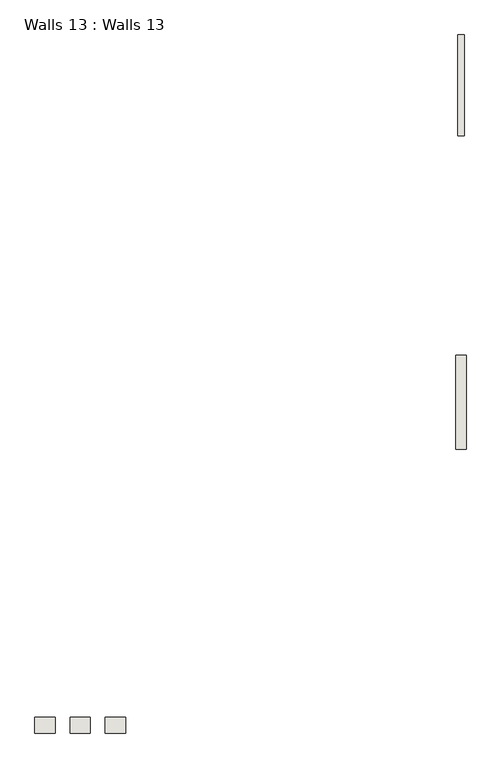
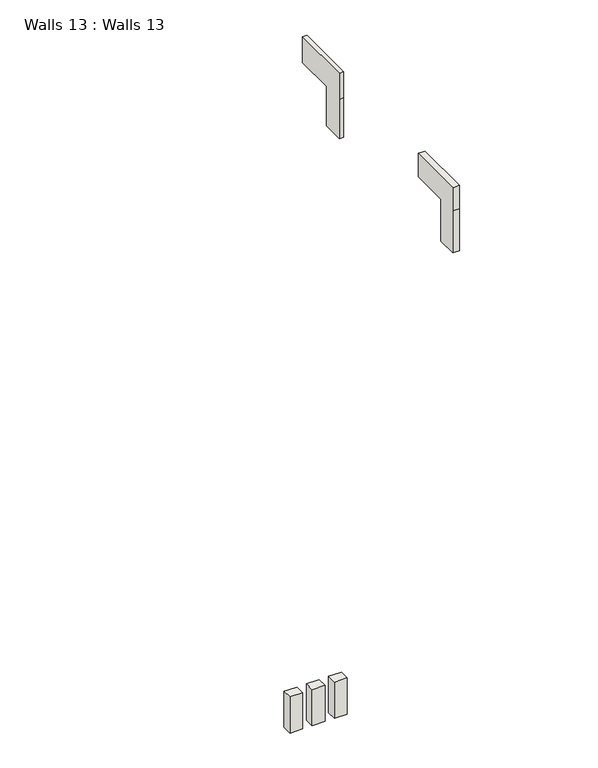
"""IFC4 building model written with IfcOpenShell, lengths in millimetres: wall geometry, Walls 13 : Walls 13."""

from ifc_helpers import new_model, si_unit, frame, origin, place, context, project, spatial, polyline, outline, extrude, source, transform, mapped, element, save


def walls_13_walls_13_75e322be(model_context):
    return source(origin(), model_context, "Body", "SweptSolid", [
        extrude(outline(polyline([(5900.1740351, 9474.2), (5900.1740351, 8820.1275419), (4918.9383511, 8820.1275419), (4918.9383511, 7820.7521516), (4376.1740351, 7820.7521516), (4376.1740351, 8820.1275419), (4376.1740351, 9474.2), (5900.1740351, 9474.2)])), frame((2302.6685091, 0.0, 0.0), z_axis=(1.0, 0.0, 0.0), x_axis=(0.0, 1.0, 0.0)), (0.0, 0.0, 1.0), 101.8221291),
        extrude(outline(polyline([(1048.7740351, 9474.2), (1048.7740351, 8885.7171315), (120.9450154, 8885.7171315), (120.9450154, 7820.7521516), (-373.6259649, 7820.7521516), (-373.6259649, 8885.7171315), (-373.6259649, 9474.2), (1048.7740351, 9474.2)])), frame((2272.4271302, 0.0, 0.0), z_axis=(1.0, 0.0, 0.0), x_axis=(0.0, 1.0, 0.0)), (0.0, 0.0, 1.0), 157.4776868),
        extrude(outline(polyline([(-3798.4727244, -4666.7213241), (-4103.2727244, -4666.7213241), (-4103.2727244, -4430.287454), (-3798.4727244, -4430.287454), (-3798.4727244, -4666.7213241)])), frame((0.0, 0.0, 519.7613395), z_axis=(0.0, 0.0, 1.0), x_axis=(1.0, 0.0, 0.0)), (0.0, 0.0, 1.0), 914.4),
        extrude(outline(polyline([(-3265.0727244, -4666.7213241), (-3569.8727244, -4666.7213241), (-3569.8727244, -4430.287454), (-3265.0727244, -4430.287454), (-3265.0727244, -4666.7213241)])), frame((0.0, 0.0, 519.7613395), z_axis=(0.0, 0.0, 1.0), x_axis=(1.0, 0.0, 0.0)), (0.0, 0.0, 1.0), 914.4),
        extrude(outline(polyline([(-2731.6727244, -4666.7213241), (-3036.4727244, -4666.7213241), (-3036.4727244, -4430.287454), (-2731.6727244, -4430.287454), (-2731.6727244, -4666.7213241)])), frame((0.0, 0.0, 519.7613395), z_axis=(0.0, 0.0, 1.0), x_axis=(1.0, 0.0, 0.0)), (0.0, 0.0, 1.0), 914.4),
    ])


if __name__ == "__main__":
    model = new_model("IFC4")
    model_context = context("Model", 3, world=origin())
    ifc_project = project(units=[si_unit("LENGTHUNIT", "METRE", prefix="MILLI")], contexts=[model_context])
    site = spatial("IfcSite", under=ifc_project)
    building = spatial("IfcBuilding", under=site)
    placement = place(None, origin())
    walls_13_walls_13_shape = walls_13_walls_13_75e322be(model_context)
    element("IfcWall", 1, ObjectType="Walls 13 : Walls 13", at=placement, inside=building, context=model_context, shape_type="MappedRepresentation", body=[
        mapped(walls_13_walls_13_shape, transform((0.0, 0.0, 0.0), x_axis=(1.0, 0.0, 0.0), y_axis=(0.0, 1.0, 0.0), z_axis=(0.0, 0.0, 1.0))),
    ])
    save(model, "model.ifc")

# Revit data of these elements
# Element 1 (IfcWall, "Walls 13 : Walls 13")
#   Materials on its faces: "Default Wall"
# Materials
#   "Default Wall": colour RGB 128 128 128, transparency 0
